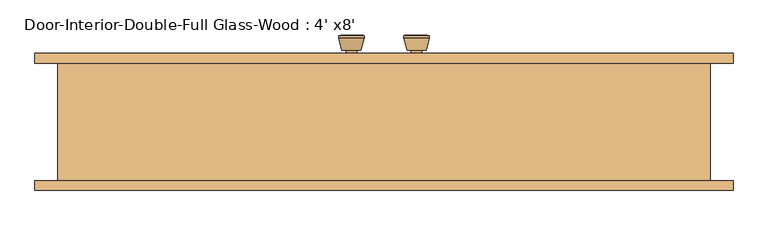
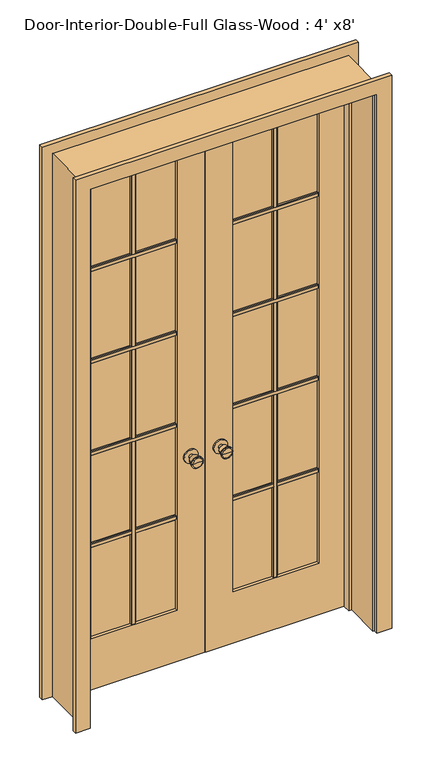
"""IFC4 building model written with IfcOpenShell, lengths in millimetres: door geometry, Door-Interior-Double-Full Glass-Wood : 4' x8'."""

from ifc_helpers import new_model, si_unit, point, frame, frame_2d, origin, place, context, project, spatial, polyline, circle_curve, trimmed, segment, composite_curve, outline, extrude, faceted_brep, source, transform, mapped, element, save
from ifc_brep_helpers import plane_surface, cylinder_surface, revolved_surface, advanced_brep


def door_interior_double_full_glass_wood_4_x8_0c92ad92(model_context):
    return source(origin(), model_context, "Body", "SolidModel", [
        advanced_brep(
        [(-63.5, 117.125, 914.4), (-73.5, 117.125, 914.4), (-53.5, 117.125, 914.4), (-83.9758676, 166.125, 914.4), (-63.5, 166.125, 914.4), (-43.0241324, 166.125, 914.4), (-88.5, 164.2971319, 914.4), (-38.5, 164.2971319, 914.4), (-88.5, 160.8334537, 914.4), (-38.5, 160.8334537, 914.4), (-82.136236, 136.125, 914.4), (-44.863764, 136.125, 914.4), (-73.5, 136.125, 914.4), (-53.5, 136.125, 914.4)],
        [
            (0, 1),
            (1, 2, circle_curve(frame((-63.5, 117.125, 914.4), z_axis=(0.0, -1.0, 0.0), x_axis=(1.0, 0.0, 0.0)), 10.0)),
            (2, 0),
            (2, 1, circle_curve(frame((-63.5, 117.125, 914.4), z_axis=(0.0, -1.0, 0.0), x_axis=(1.0, 0.0, 0.0)), 10.0)),
            (3, 4),
            (4, 5),
            (5, 3, circle_curve(frame((-63.5, 166.125, 914.4), z_axis=(0.0, 1.0, 0.0), x_axis=(1.0, 0.0, 0.0)), 20.4758676)),
            (3, 5, circle_curve(frame((-63.5, 166.125, 914.4), z_axis=(0.0, 1.0, 0.0), x_axis=(1.0, 0.0, 0.0)), 20.4758676)),
            (6, 3),
            (5, 7),
            (7, 6, circle_curve(frame((-63.5, 164.2971319, 914.4), z_axis=(0.0, 1.0, 0.0), x_axis=(1.0, 0.0, 0.0)), 25.0)),
            (6, 7, circle_curve(frame((-63.5, 164.2971319, 914.4), z_axis=(0.0, 1.0, 0.0), x_axis=(1.0, 0.0, 0.0)), 25.0)),
            (8, 6),
            (7, 9),
            (9, 8, circle_curve(frame((-63.5, 160.8334537, 914.4), z_axis=(0.0, 1.0, 0.0), x_axis=(1.0, 0.0, 0.0)), 25.0)),
            (8, 9, circle_curve(frame((-63.5, 160.8334537, 914.4), z_axis=(0.0, 1.0, 0.0), x_axis=(1.0, 0.0, 0.0)), 25.0)),
            (10, 8),
            (9, 11),
            (11, 10, circle_curve(frame((-63.5, 136.125, 914.4), z_axis=(0.0, 1.0, 0.0), x_axis=(1.0, 0.0, 0.0)), 18.636236)),
            (10, 11, circle_curve(frame((-63.5, 136.125, 914.4), z_axis=(0.0, 1.0, 0.0), x_axis=(1.0, 0.0, 0.0)), 18.636236)),
            (12, 10),
            (11, 13),
            (13, 12, circle_curve(frame((-63.5, 136.125, 914.4), z_axis=(0.0, 1.0, 0.0), x_axis=(1.0, 0.0, 0.0)), 10.0)),
            (12, 13, circle_curve(frame((-63.5, 136.125, 914.4), z_axis=(0.0, 1.0, 0.0), x_axis=(1.0, 0.0, 0.0)), 10.0)),
            (1, 12),
            (13, 2),
        ],
        [
            plane_surface(frame((-63.5, 117.125, 914.4), z_axis=(0.0, -1.0, 0.0), x_axis=(1.0, 0.0, 0.0))),
            plane_surface(frame((-63.5, 166.125, 914.4), z_axis=(0.0, 1.0, 0.0), x_axis=(1.0, 0.0, 0.0))),
            revolved_surface(polyline([(-43.0241324, 166.125, 914.4), (-38.5, 164.2971319, 914.4)]), (-63.5, 117.125, 914.4), (0.0, -1.0, 0.0)),
            cylinder_surface(frame((-63.5, 117.125, 914.4), z_axis=(0.0, -1.0, 0.0), x_axis=(1.0, 0.0, 0.0)), 25.0),
            revolved_surface(polyline([(-38.5, 160.8334537, 914.4), (-44.863764, 136.125, 914.4)]), (-63.5, 117.125, 914.4), (0.0, -1.0, 0.0)),
            plane_surface(frame((-63.5, 136.125, 914.4), z_axis=(0.0, -1.0, 0.0), x_axis=(1.0, 0.0, 0.0))),
            cylinder_surface(frame((-63.5, 117.125, 914.4), z_axis=(0.0, -1.0, 0.0), x_axis=(1.0, 0.0, 0.0)), 10.0),
        ],
        [
            (0, [[1, 2, 3]]),
            (0, [[-3, 4, -1]]),
            (1, [[5, 6, 7]]),
            (1, [[-6, -5, 8]]),
            (2, [[9, -7, 10, 11]]),
            (2, [[-10, -8, -9, 12]]),
            (3, [[13, -11, 14, 15]]),
            (3, [[-14, -12, -13, 16]]),
            (4, [[17, -15, 18, 19]]),
            (4, [[-18, -16, -17, 20]]),
            (5, [[21, -19, 22, 23]]),
            (5, [[-22, -20, -21, 24]]),
            (6, [[25, -23, 26, -2]]),
            (6, [[-26, -24, -25, -4]]),
        ],
    ),
        extrude(outline(composite_curve([segment(trimmed(circle_curve(frame_2d((914.4, -63.5)), 30.0), [point((914.4, -33.5))], [point((914.4, -93.5))], False, "CARTESIAN"), True, "CONTINUOUS"), segment(trimmed(circle_curve(frame_2d((914.4, -63.5)), 30.0), [point((914.4, -93.5))], [point((914.4, -33.5))], False, "CARTESIAN"), True, "CONTINUOUS")], self_intersect=False)), frame((0.0, 111.125, 0.0), z_axis=(0.0, 1.0, 0.0), x_axis=(0.0, 0.0, 1.0)), (0.0, 0.0, 1.0), 6.0),
        advanced_brep(
        [(-63.5, 70.2, 914.4), (-53.5, 70.2, 914.4), (-73.5, 70.2, 914.4), (-83.9758676, 21.2, 914.4), (-43.0241324, 21.2, 914.4), (-63.5, 21.2, 914.4), (-88.5, 23.0278681, 914.4), (-38.5, 23.0278681, 914.4), (-88.5, 26.4915463, 914.4), (-38.5, 26.4915463, 914.4), (-82.136236, 51.2, 914.4), (-44.863764, 51.2, 914.4), (-73.5, 51.2, 914.4), (-53.5, 51.2, 914.4)],
        [
            (0, 1),
            (1, 2, circle_curve(frame((-63.5, 70.2, 914.4), z_axis=(0.0, 1.0, 0.0), x_axis=(1.0, 0.0, 0.0)), 10.0)),
            (2, 0),
            (2, 1, circle_curve(frame((-63.5, 70.2, 914.4), z_axis=(0.0, 1.0, 0.0), x_axis=(1.0, 0.0, 0.0)), 10.0)),
            (3, 4, circle_curve(frame((-63.5, 21.2, 914.4), z_axis=(0.0, -1.0, 0.0), x_axis=(1.0, 0.0, 0.0)), 20.4758676)),
            (4, 5),
            (5, 3),
            (4, 3, circle_curve(frame((-63.5, 21.2, 914.4), z_axis=(0.0, -1.0, 0.0), x_axis=(1.0, 0.0, 0.0)), 20.4758676)),
            (6, 7, circle_curve(frame((-63.5, 23.0278681, 914.4), z_axis=(0.0, -1.0, 0.0), x_axis=(1.0, 0.0, 0.0)), 25.0)),
            (7, 4),
            (3, 6),
            (7, 6, circle_curve(frame((-63.5, 23.0278681, 914.4), z_axis=(0.0, -1.0, 0.0), x_axis=(1.0, 0.0, 0.0)), 25.0)),
            (8, 9, circle_curve(frame((-63.5, 26.4915463, 914.4), z_axis=(0.0, -1.0, 0.0), x_axis=(1.0, 0.0, 0.0)), 25.0)),
            (9, 7),
            (6, 8),
            (9, 8, circle_curve(frame((-63.5, 26.4915463, 914.4), z_axis=(0.0, -1.0, 0.0), x_axis=(1.0, 0.0, 0.0)), 25.0)),
            (10, 11, circle_curve(frame((-63.5, 51.2, 914.4), z_axis=(0.0, -1.0, 0.0), x_axis=(1.0, 0.0, 0.0)), 18.636236)),
            (11, 9),
            (8, 10),
            (11, 10, circle_curve(frame((-63.5, 51.2, 914.4), z_axis=(0.0, -1.0, 0.0), x_axis=(1.0, 0.0, 0.0)), 18.636236)),
            (12, 13, circle_curve(frame((-63.5, 51.2, 914.4), z_axis=(0.0, -1.0, 0.0), x_axis=(1.0, 0.0, 0.0)), 10.0)),
            (13, 11),
            (10, 12),
            (13, 12, circle_curve(frame((-63.5, 51.2, 914.4), z_axis=(0.0, -1.0, 0.0), x_axis=(1.0, 0.0, 0.0)), 10.0)),
            (1, 13),
            (12, 2),
        ],
        [
            plane_surface(frame((-63.5, 70.2, 914.4), z_axis=(0.0, 1.0, 0.0), x_axis=(1.0, 0.0, 0.0))),
            plane_surface(frame((-63.5, 21.2, 914.4), z_axis=(0.0, -1.0, 0.0), x_axis=(1.0, 0.0, 0.0))),
            revolved_surface(polyline([(-43.0241324, 21.2, 914.4), (-38.5, 23.0278681, 914.4)]), (-63.5, 70.2, 914.4), (0.0, 1.0, 0.0)),
            cylinder_surface(frame((-63.5, 70.2, 914.4), z_axis=(0.0, 1.0, 0.0), x_axis=(1.0, 0.0, 0.0)), 25.0),
            revolved_surface(polyline([(-38.5, 26.4915463, 914.4), (-44.863764, 51.2, 914.4)]), (-63.5, 70.2, 914.4), (0.0, 1.0, 0.0)),
            plane_surface(frame((-63.5, 51.2, 914.4), z_axis=(0.0, 1.0, 0.0), x_axis=(1.0, 0.0, 0.0))),
            cylinder_surface(frame((-63.5, 70.2, 914.4), z_axis=(0.0, 1.0, 0.0), x_axis=(1.0, 0.0, 0.0)), 10.0),
        ],
        [
            (0, [[1, 2, 3]]),
            (0, [[-3, 4, -1]]),
            (1, [[5, 6, 7]]),
            (1, [[8, -7, -6]]),
            (2, [[9, 10, -5, 11]]),
            (2, [[12, -11, -8, -10]]),
            (3, [[13, 14, -9, 15]]),
            (3, [[16, -15, -12, -14]]),
            (4, [[17, 18, -13, 19]]),
            (4, [[20, -19, -16, -18]]),
            (5, [[21, 22, -17, 23]]),
            (5, [[24, -23, -20, -22]]),
            (6, [[-2, 25, -21, 26]]),
            (6, [[-4, -26, -24, -25]]),
        ],
    ),
        extrude(outline(composite_curve([segment(trimmed(circle_curve(frame_2d((914.4, -63.5)), 30.0), [point((914.4, -33.5))], [point((914.4, -93.5))], False, "CARTESIAN"), True, "CONTINUOUS"), segment(trimmed(circle_curve(frame_2d((914.4, -63.5)), 30.0), [point((914.4, -93.5))], [point((914.4, -33.5))], False, "CARTESIAN"), True, "CONTINUOUS")], self_intersect=False)), frame((0.0, 70.2, 0.0), z_axis=(0.0, 1.0, 0.0), x_axis=(0.0, 0.0, 1.0)), (0.0, 0.0, 1.0), 6.0),
        extrude(outline(polyline([(90.17, 1911.35), (90.17, 1892.3), (83.82, 1892.3), (80.645, 1895.475), (80.645, 1908.175), (83.82, 1911.35), (90.17, 1911.35)])), frame((120.65, 0.0, 0.0), z_axis=(1.0, 0.0, 0.0), x_axis=(0.0, 1.0, 0.0)), (0.0, 0.0, 1.0), 368.3),
        extrude(outline(polyline([(90.17, 1493.8375), (90.17, 1474.7875), (83.82, 1474.7875), (80.645, 1477.9625), (80.645, 1490.6625), (83.82, 1493.8375), (90.17, 1493.8375)])), frame((120.65, 0.0, 0.0), z_axis=(1.0, 0.0, 0.0), x_axis=(0.0, 1.0, 0.0)), (0.0, 0.0, 1.0), 368.3),
        extrude(outline(polyline([(90.17, 1076.325), (90.17, 1057.275), (83.82, 1057.275), (80.645, 1060.45), (80.645, 1073.15), (83.82, 1076.325), (90.17, 1076.325)])), frame((120.65, 0.0, 0.0), z_axis=(1.0, 0.0, 0.0), x_axis=(0.0, 1.0, 0.0)), (0.0, 0.0, 1.0), 368.3),
        extrude(outline(polyline([(295.275, 90.17), (314.325, 90.17), (314.325, 83.82), (311.15, 80.645), (298.45, 80.645), (295.275, 83.82), (295.275, 90.17)])), frame((0.0, 0.0, 231.775), z_axis=(0.0, 0.0, 1.0), x_axis=(1.0, 0.0, 0.0)), (0.0, 0.0, 1.0), 2087.5625),
        extrude(outline(polyline([(90.17, 658.8125), (90.17, 639.7625), (83.82, 639.7625), (80.645, 642.9375), (80.645, 655.6375), (83.82, 658.8125), (90.17, 658.8125)])), frame((120.65, 0.0, 0.0), z_axis=(1.0, 0.0, 0.0), x_axis=(0.0, 1.0, 0.0)), (0.0, 0.0, 1.0), 368.3),
        extrude(outline(polyline([(97.155, 1911.35), (103.505, 1911.35), (106.68, 1908.175), (106.68, 1895.475), (103.505, 1892.3), (97.155, 1892.3), (97.155, 1911.35)])), frame((-488.95, 0.0, 0.0), z_axis=(1.0, 0.0, 0.0), x_axis=(0.0, 1.0, 0.0)), (0.0, 0.0, 1.0), 368.3),
        extrude(outline(polyline([(97.155, 1493.8375), (103.505, 1493.8375), (106.68, 1490.6625), (106.68, 1477.9625), (103.505, 1474.7875), (97.155, 1474.7875), (97.155, 1493.8375)])), frame((-488.95, 0.0, 0.0), z_axis=(1.0, 0.0, 0.0), x_axis=(0.0, 1.0, 0.0)), (0.0, 0.0, 1.0), 368.3),
        extrude(outline(polyline([(97.155, 1076.325), (103.505, 1076.325), (106.68, 1073.15), (106.68, 1060.45), (103.505, 1057.275), (97.155, 1057.275), (97.155, 1076.325)])), frame((-488.95, 0.0, 0.0), z_axis=(1.0, 0.0, 0.0), x_axis=(0.0, 1.0, 0.0)), (0.0, 0.0, 1.0), 368.3),
        extrude(outline(polyline([(-314.325, 97.155), (-314.325, 103.505), (-311.15, 106.68), (-298.45, 106.68), (-295.275, 103.505), (-295.275, 97.155), (-314.325, 97.155)])), frame((0.0, 0.0, 231.775), z_axis=(0.0, 0.0, 1.0), x_axis=(1.0, 0.0, 0.0)), (0.0, 0.0, 1.0), 2087.5625),
        extrude(outline(polyline([(97.155, 658.8125), (103.505, 658.8125), (106.68, 655.6375), (106.68, 642.9375), (103.505, 639.7625), (97.155, 639.7625), (97.155, 658.8125)])), frame((-488.95, 0.0, 0.0), z_axis=(1.0, 0.0, 0.0), x_axis=(0.0, 1.0, 0.0)), (0.0, 0.0, 1.0), 368.3),
        extrude(outline(polyline([(97.155, 1911.35), (103.505, 1911.35), (106.68, 1908.175), (106.68, 1895.475), (103.505, 1892.3), (97.155, 1892.3), (97.155, 1911.35)])), frame((120.65, 0.0, 0.0), z_axis=(1.0, 0.0, 0.0), x_axis=(0.0, 1.0, 0.0)), (0.0, 0.0, 1.0), 368.3),
        extrude(outline(polyline([(97.155, 1493.8375), (103.505, 1493.8375), (106.68, 1490.6625), (106.68, 1477.9625), (103.505, 1474.7875), (97.155, 1474.7875), (97.155, 1493.8375)])), frame((120.65, 0.0, 0.0), z_axis=(1.0, 0.0, 0.0), x_axis=(0.0, 1.0, 0.0)), (0.0, 0.0, 1.0), 368.3),
        extrude(outline(polyline([(97.155, 1076.325), (103.505, 1076.325), (106.68, 1073.15), (106.68, 1060.45), (103.505, 1057.275), (97.155, 1057.275), (97.155, 1076.325)])), frame((120.65, 0.0, 0.0), z_axis=(1.0, 0.0, 0.0), x_axis=(0.0, 1.0, 0.0)), (0.0, 0.0, 1.0), 368.3),
        extrude(outline(polyline([(295.275, 97.155), (295.275, 103.505), (298.45, 106.68), (311.15, 106.68), (314.325, 103.505), (314.325, 97.155), (295.275, 97.155)])), frame((0.0, 0.0, 231.775), z_axis=(0.0, 0.0, 1.0), x_axis=(1.0, 0.0, 0.0)), (0.0, 0.0, 1.0), 2087.5625),
        extrude(outline(polyline([(97.155, 658.8125), (103.505, 658.8125), (106.68, 655.6375), (106.68, 642.9375), (103.505, 639.7625), (97.155, 639.7625), (97.155, 658.8125)])), frame((120.65, 0.0, 0.0), z_axis=(1.0, 0.0, 0.0), x_axis=(0.0, 1.0, 0.0)), (0.0, 0.0, 1.0), 368.3),
        extrude(outline(polyline([(90.17, 1911.35), (90.17, 1892.3), (83.82, 1892.3), (80.645, 1895.475), (80.645, 1908.175), (83.82, 1911.35), (90.17, 1911.35)])), frame((-488.95, 0.0, 0.0), z_axis=(1.0, 0.0, 0.0), x_axis=(0.0, 1.0, 0.0)), (0.0, 0.0, 1.0), 368.3),
        extrude(outline(polyline([(90.17, 1493.8375), (90.17, 1474.7875), (83.82, 1474.7875), (80.645, 1477.9625), (80.645, 1490.6625), (83.82, 1493.8375), (90.17, 1493.8375)])), frame((-488.95, 0.0, 0.0), z_axis=(1.0, 0.0, 0.0), x_axis=(0.0, 1.0, 0.0)), (0.0, 0.0, 1.0), 368.3),
        extrude(outline(polyline([(90.17, 1076.325), (90.17, 1057.275), (83.82, 1057.275), (80.645, 1060.45), (80.645, 1073.15), (83.82, 1076.325), (90.17, 1076.325)])), frame((-488.95, 0.0, 0.0), z_axis=(1.0, 0.0, 0.0), x_axis=(0.0, 1.0, 0.0)), (0.0, 0.0, 1.0), 368.3),
        extrude(outline(polyline([(-314.325, 90.17), (-295.275, 90.17), (-295.275, 83.82), (-298.45, 80.645), (-311.15, 80.645), (-314.325, 83.82), (-314.325, 90.17)])), frame((0.0, 0.0, 231.775), z_axis=(0.0, 0.0, 1.0), x_axis=(1.0, 0.0, 0.0)), (0.0, 0.0, 1.0), 2087.5625),
        extrude(outline(polyline([(90.17, 658.8125), (90.17, 639.7625), (83.82, 639.7625), (80.645, 642.9375), (80.645, 655.6375), (83.82, 658.8125), (90.17, 658.8125)])), frame((-488.95, 0.0, 0.0), z_axis=(1.0, 0.0, 0.0), x_axis=(0.0, 1.0, 0.0)), (0.0, 0.0, 1.0), 368.3),
        advanced_brep(
        [(63.5, 70.2, 914.4), (73.5, 70.2, 914.4), (53.5, 70.2, 914.4), (83.9758676, 21.2, 914.4), (63.5, 21.2, 914.4), (43.0241324, 21.2, 914.4), (88.5, 23.0278681, 914.4), (38.5, 23.0278681, 914.4), (88.5, 26.4915463, 914.4), (38.5, 26.4915463, 914.4), (82.136236, 51.2, 914.4), (44.863764, 51.2, 914.4), (73.5, 51.2, 914.4), (53.5, 51.2, 914.4)],
        [
            (0, 1),
            (1, 2, circle_curve(frame((63.5, 70.2, 914.4), z_axis=(0.0, 1.0, 0.0), x_axis=(-1.0, 0.0, 0.0)), 10.0)),
            (2, 0),
            (2, 1, circle_curve(frame((63.5, 70.2, 914.4), z_axis=(0.0, 1.0, 0.0), x_axis=(-1.0, 0.0, 0.0)), 10.0)),
            (3, 4),
            (4, 5),
            (5, 3, circle_curve(frame((63.5, 21.2, 914.4), z_axis=(0.0, -1.0, 0.0), x_axis=(-1.0, 0.0, 0.0)), 20.4758676)),
            (3, 5, circle_curve(frame((63.5, 21.2, 914.4), z_axis=(0.0, -1.0, 0.0), x_axis=(-1.0, 0.0, 0.0)), 20.4758676)),
            (6, 3),
            (5, 7),
            (7, 6, circle_curve(frame((63.5, 23.0278681, 914.4), z_axis=(0.0, -1.0, 0.0), x_axis=(-1.0, 0.0, 0.0)), 25.0)),
            (6, 7, circle_curve(frame((63.5, 23.0278681, 914.4), z_axis=(0.0, -1.0, 0.0), x_axis=(-1.0, 0.0, 0.0)), 25.0)),
            (8, 6),
            (7, 9),
            (9, 8, circle_curve(frame((63.5, 26.4915463, 914.4), z_axis=(0.0, -1.0, 0.0), x_axis=(-1.0, 0.0, 0.0)), 25.0)),
            (8, 9, circle_curve(frame((63.5, 26.4915463, 914.4), z_axis=(0.0, -1.0, 0.0), x_axis=(-1.0, 0.0, 0.0)), 25.0)),
            (10, 8),
            (9, 11),
            (11, 10, circle_curve(frame((63.5, 51.2, 914.4), z_axis=(0.0, -1.0, 0.0), x_axis=(-1.0, 0.0, 0.0)), 18.636236)),
            (10, 11, circle_curve(frame((63.5, 51.2, 914.4), z_axis=(0.0, -1.0, 0.0), x_axis=(-1.0, 0.0, 0.0)), 18.636236)),
            (12, 10),
            (11, 13),
            (13, 12, circle_curve(frame((63.5, 51.2, 914.4), z_axis=(0.0, -1.0, 0.0), x_axis=(-1.0, 0.0, 0.0)), 10.0)),
            (12, 13, circle_curve(frame((63.5, 51.2, 914.4), z_axis=(0.0, -1.0, 0.0), x_axis=(-1.0, 0.0, 0.0)), 10.0)),
            (1, 12),
            (13, 2),
        ],
        [
            plane_surface(frame((63.5, 70.2, 914.4), z_axis=(0.0, 1.0, 0.0), x_axis=(-1.0, 0.0, 0.0))),
            plane_surface(frame((63.5, 21.2, 914.4), z_axis=(0.0, -1.0, 0.0), x_axis=(-1.0, 0.0, 0.0))),
            revolved_surface(polyline([(43.0241324, 21.2, 914.4), (38.5, 23.0278681, 914.4)]), (63.5, 70.2, 914.4), (0.0, 1.0, 0.0)),
            cylinder_surface(frame((63.5, 70.2, 914.4), z_axis=(0.0, 1.0, 0.0), x_axis=(-1.0, 0.0, 0.0)), 25.0),
            revolved_surface(polyline([(38.5, 26.4915463, 914.4), (44.863764, 51.2, 914.4)]), (63.5, 70.2, 914.4), (0.0, 1.0, 0.0)),
            plane_surface(frame((63.5, 51.2, 914.4), z_axis=(0.0, 1.0, 0.0), x_axis=(-1.0, 0.0, 0.0))),
            cylinder_surface(frame((63.5, 70.2, 914.4), z_axis=(0.0, 1.0, 0.0), x_axis=(-1.0, 0.0, 0.0)), 10.0),
        ],
        [
            (0, [[1, 2, 3]]),
            (0, [[-3, 4, -1]]),
            (1, [[5, 6, 7]]),
            (1, [[-6, -5, 8]]),
            (2, [[9, -7, 10, 11]]),
            (2, [[-10, -8, -9, 12]]),
            (3, [[13, -11, 14, 15]]),
            (3, [[-14, -12, -13, 16]]),
            (4, [[17, -15, 18, 19]]),
            (4, [[-18, -16, -17, 20]]),
            (5, [[21, -19, 22, 23]]),
            (5, [[-22, -20, -21, 24]]),
            (6, [[25, -23, 26, -2]]),
            (6, [[-26, -24, -25, -4]]),
        ],
    ),
        extrude(outline(composite_curve([segment(trimmed(circle_curve(frame_2d((914.4, 63.5)), 30.0), [point((914.4, 33.5))], [point((914.4, 93.5))], False, "CARTESIAN"), True, "CONTINUOUS"), segment(trimmed(circle_curve(frame_2d((914.4, 63.5)), 30.0), [point((914.4, 93.5))], [point((914.4, 33.5))], False, "CARTESIAN"), True, "CONTINUOUS")], self_intersect=False)), frame((0.0, 70.2, 0.0), z_axis=(0.0, 1.0, 0.0), x_axis=(0.0, 0.0, 1.0)), (0.0, 0.0, 1.0), 6.0),
        advanced_brep(
        [(63.5, 117.125, 914.4), (53.5, 117.125, 914.4), (73.5, 117.125, 914.4), (83.9758676, 166.125, 914.4), (43.0241324, 166.125, 914.4), (63.5, 166.125, 914.4), (88.5, 164.2971319, 914.4), (38.5, 164.2971319, 914.4), (88.5, 160.8334537, 914.4), (38.5, 160.8334537, 914.4), (82.136236, 136.125, 914.4), (44.863764, 136.125, 914.4), (73.5, 136.125, 914.4), (53.5, 136.125, 914.4)],
        [
            (0, 1),
            (1, 2, circle_curve(frame((63.5, 117.125, 914.4), z_axis=(0.0, -1.0, 0.0), x_axis=(-1.0, 0.0, 0.0)), 10.0)),
            (2, 0),
            (2, 1, circle_curve(frame((63.5, 117.125, 914.4), z_axis=(0.0, -1.0, 0.0), x_axis=(-1.0, 0.0, 0.0)), 10.0)),
            (3, 4, circle_curve(frame((63.5, 166.125, 914.4), z_axis=(0.0, 1.0, 0.0), x_axis=(-1.0, 0.0, 0.0)), 20.4758676)),
            (4, 5),
            (5, 3),
            (4, 3, circle_curve(frame((63.5, 166.125, 914.4), z_axis=(0.0, 1.0, 0.0), x_axis=(-1.0, 0.0, 0.0)), 20.4758676)),
            (6, 7, circle_curve(frame((63.5, 164.2971319, 914.4), z_axis=(0.0, 1.0, 0.0), x_axis=(-1.0, 0.0, 0.0)), 25.0)),
            (7, 4),
            (3, 6),
            (7, 6, circle_curve(frame((63.5, 164.2971319, 914.4), z_axis=(0.0, 1.0, 0.0), x_axis=(-1.0, 0.0, 0.0)), 25.0)),
            (8, 9, circle_curve(frame((63.5, 160.8334537, 914.4), z_axis=(0.0, 1.0, 0.0), x_axis=(-1.0, 0.0, 0.0)), 25.0)),
            (9, 7),
            (6, 8),
            (9, 8, circle_curve(frame((63.5, 160.8334537, 914.4), z_axis=(0.0, 1.0, 0.0), x_axis=(-1.0, 0.0, 0.0)), 25.0)),
            (10, 11, circle_curve(frame((63.5, 136.125, 914.4), z_axis=(0.0, 1.0, 0.0), x_axis=(-1.0, 0.0, 0.0)), 18.636236)),
            (11, 9),
            (8, 10),
            (11, 10, circle_curve(frame((63.5, 136.125, 914.4), z_axis=(0.0, 1.0, 0.0), x_axis=(-1.0, 0.0, 0.0)), 18.636236)),
            (12, 13, circle_curve(frame((63.5, 136.125, 914.4), z_axis=(0.0, 1.0, 0.0), x_axis=(-1.0, 0.0, 0.0)), 10.0)),
            (13, 11),
            (10, 12),
            (13, 12, circle_curve(frame((63.5, 136.125, 914.4), z_axis=(0.0, 1.0, 0.0), x_axis=(-1.0, 0.0, 0.0)), 10.0)),
            (1, 13),
            (12, 2),
        ],
        [
            plane_surface(frame((63.5, 117.125, 914.4), z_axis=(0.0, -1.0, 0.0), x_axis=(-1.0, 0.0, 0.0))),
            plane_surface(frame((63.5, 166.125, 914.4), z_axis=(0.0, 1.0, 0.0), x_axis=(-1.0, 0.0, 0.0))),
            revolved_surface(polyline([(43.0241324, 166.125, 914.4), (38.5, 164.2971319, 914.4)]), (63.5, 117.125, 914.4), (0.0, -1.0, 0.0)),
            cylinder_surface(frame((63.5, 117.125, 914.4), z_axis=(0.0, -1.0, 0.0), x_axis=(-1.0, 0.0, 0.0)), 25.0),
            revolved_surface(polyline([(38.5, 160.8334537, 914.4), (44.863764, 136.125, 914.4)]), (63.5, 117.125, 914.4), (0.0, -1.0, 0.0)),
            plane_surface(frame((63.5, 136.125, 914.4), z_axis=(0.0, -1.0, 0.0), x_axis=(-1.0, 0.0, 0.0))),
            cylinder_surface(frame((63.5, 117.125, 914.4), z_axis=(0.0, -1.0, 0.0), x_axis=(-1.0, 0.0, 0.0)), 10.0),
        ],
        [
            (0, [[1, 2, 3]]),
            (0, [[-3, 4, -1]]),
            (1, [[5, 6, 7]]),
            (1, [[8, -7, -6]]),
            (2, [[9, 10, -5, 11]]),
            (2, [[12, -11, -8, -10]]),
            (3, [[13, 14, -9, 15]]),
            (3, [[16, -15, -12, -14]]),
            (4, [[17, 18, -13, 19]]),
            (4, [[20, -19, -16, -18]]),
            (5, [[21, 22, -17, 23]]),
            (5, [[24, -23, -20, -22]]),
            (6, [[-2, 25, -21, 26]]),
            (6, [[-4, -26, -24, -25]]),
        ],
    ),
        extrude(outline(composite_curve([segment(trimmed(circle_curve(frame_2d((914.4, 63.5)), 30.0), [point((914.4, 33.5))], [point((914.4, 93.5))], False, "CARTESIAN"), True, "CONTINUOUS"), segment(trimmed(circle_curve(frame_2d((914.4, 63.5)), 30.0), [point((914.4, 93.5))], [point((914.4, 33.5))], False, "CARTESIAN"), True, "CONTINUOUS")], self_intersect=False)), frame((0.0, 111.125, 0.0), z_axis=(0.0, 1.0, 0.0), x_axis=(0.0, 0.0, 1.0)), (0.0, 0.0, 1.0), 6.0),
        extrude(outline(polyline([(0.0, 615.95), (0.0, 679.45), (2508.25, 679.45), (2508.25, -679.45), (0.0, -679.45), (0.0, -615.95), (2444.75, -615.95), (2444.75, 615.95), (0.0, 615.95)])), frame((0.0, -136.525, 0.0), z_axis=(0.0, 1.0, 0.0), x_axis=(0.0, 0.0, 1.0)), (0.0, 0.0, 1.0), 19.05),
        extrude(outline(polyline([(0.0, 615.95), (0.0, 679.45), (2508.25, 679.45), (2508.25, -679.45), (0.0, -679.45), (0.0, -615.95), (2444.75, -615.95), (2444.75, 615.95), (0.0, 615.95)])), frame((0.0, 111.125, 0.0), z_axis=(0.0, 1.0, 0.0), x_axis=(0.0, 0.0, 1.0)), (0.0, 0.0, 1.0), 19.05),
        faceted_brep([(635.0, 111.125, 0.0), (635.0, -117.475, 0.0), (609.6, -117.475, 0.0), (609.6, 41.275, 0.0), (596.9, 41.275, 0.0), (596.9, 76.2, 0.0), (609.6, 76.2, 0.0), (609.6, 111.125, 0.0), (635.0, 111.125, 2463.8), (635.0, -117.475, 2463.8), (-635.0, -117.475, 2463.8), (-635.0, -117.475, 0.0), (-609.6, -117.475, 0.0), (-609.6, -117.475, 2438.4), (609.6, -117.475, 2438.4), (609.6, 41.275, 2438.4), (-609.6, 41.275, 2438.4), (-609.6, 41.275, 0.0), (-596.9, 41.275, 0.0), (-596.9, 41.275, 2425.7), (596.9, 41.275, 2425.7), (596.9, 76.2, 2425.7), (1.5875, 76.2, 2425.7), (-1.6019111, 76.2, 2425.7), (-596.9, 76.2, 2425.7), (-596.9, 76.2, 0.0), (-609.6, 76.2, 0.0), (-609.6, 76.2, 2438.4), (-1.6019111, 76.2, 2438.4), (1.5875, 76.2, 2438.4), (609.6, 76.2, 2438.4), (609.6, 111.125, 2438.4), (1.5875, 111.125, 2438.4), (-1.6019111, 111.125, 2438.4), (-609.6, 111.125, 2438.4), (-609.6, 111.125, 0.0), (-635.0, 111.125, 0.0), (-635.0, 111.125, 2463.8)], [[[0, 1, 2, 3, 4, 5, 6, 7]], [[1, 0, 8, 9]], [[2, 1, 9, 10, 11, 12, 13, 14]], [[3, 2, 14, 15]], [[4, 3, 15, 16, 17, 18, 19, 20]], [[5, 4, 20, 21]], [[6, 5, 21, 22, 23, 24, 25, 26, 27, 28, 29, 30]], [[7, 6, 30, 31]], [[0, 7, 31, 32, 33, 34, 35, 36, 37, 8]], [[9, 8, 37, 10]], [[14, 13, 16, 15]], [[20, 19, 24, 23, 22, 21]], [[31, 30, 29, 28, 27, 34, 33, 32]], [[12, 11, 36, 35, 26, 25, 18, 17]], [[11, 10, 37, 36]], [[13, 12, 17, 16]], [[19, 18, 25, 24]], [[27, 26, 35, 34]]]),
        extrude(outline(polyline([(2438.4, -609.6), (0.0, -609.6), (0.0, -1.6019111), (2438.4, -1.6019111), (2438.4, -609.6)]), holes=[polyline([(231.775, -488.95), (2319.3375, -488.95), (2319.3375, -120.65), (231.775, -120.65), (231.775, -488.95)])]), frame((0.0, 76.2, 0.0), z_axis=(0.0, 1.0, 0.0), x_axis=(0.0, 0.0, 1.0)), (0.0, 0.0, 1.0), 34.925),
        extrude(outline(polyline([(0.0, 609.6), (2438.4, 609.6), (2438.4, 1.5875), (0.0, 1.5875), (0.0, 609.6)]), holes=[polyline([(2319.3375, 120.65), (2319.3375, 488.95), (231.775, 488.95), (231.775, 120.65), (2319.3375, 120.65)])]), frame((0.0, 76.2, 0.0), z_axis=(0.0, 1.0, 0.0), x_axis=(0.0, 0.0, 1.0)), (0.0, 0.0, 1.0), 34.925),
        extrude(outline(polyline([(488.95, 90.17), (120.65, 90.17), (120.65, 97.155), (488.95, 97.155), (488.95, 90.17)])), frame((0.0, 0.0, 231.775), z_axis=(0.0, 0.0, 1.0), x_axis=(1.0, 0.0, 0.0)), (0.0, 0.0, 1.0), 2087.5625),
        extrude(outline(polyline([(-120.65, 90.17), (-488.95, 90.17), (-488.95, 97.155), (-120.65, 97.155), (-120.65, 90.17)])), frame((0.0, 0.0, 231.775), z_axis=(0.0, 0.0, 1.0), x_axis=(1.0, 0.0, 0.0)), (0.0, 0.0, 1.0), 2087.5625),
    ])


if __name__ == "__main__":
    model = new_model("IFC4")
    model_context = context("Model", 3, world=origin())
    ifc_project = project(units=[si_unit("LENGTHUNIT", "METRE", prefix="MILLI")], contexts=[model_context])
    site = spatial("IfcSite", under=ifc_project)
    building = spatial("IfcBuilding", under=site)
    placement = place(None, origin())
    door_interior_double_full_glass_wood_4_x8_shape = door_interior_double_full_glass_wood_4_x8_0c92ad92(model_context)
    element("IfcDoor", 1, ObjectType="Door-Interior-Double-Full Glass-Wood : 4' x8'", at=placement, inside=building, context=model_context, shape_type="MappedRepresentation", body=[
        mapped(door_interior_double_full_glass_wood_4_x8_shape, transform((0.0, 0.0, 0.0), x_axis=(1.0, 0.0, 0.0), y_axis=(0.0, 1.0, 0.0), z_axis=(0.0, 0.0, 1.0))),
    ])
    save(model, "model.ifc")

# Revit data of these elements
# Type "Door-Interior-Double-Full Glass-Wood : 4' x8'"
#   Type Mark = "14"
#   Assembly Code = "C1020300"
#   Analytic Construction = "French door, wood frame with single glass"
#   Top Rail = 0' - 4 11/16"
#   Thickness = 0' - 1 3/8"
#   Thermal Resistance (R) = 1.0696 (h·ft²·°F)/BTU
#   Swing Angle [instance default] = 90.00°
#   Stiles = 0' - 4 3/4"
#   Rough Width = 4' - 2"
#   Rough Height = 8' - 1"
#   Panel Width = 2' - 0"
#   Height = 8' - 0"
#   Width = 4' - 0"
#   Heat Transfer Coefficient (U) = 0.9350 BTU/(h·ft²·°F)
#   Bottom Rail = 0' - 9 1/8"
#   Show Grill [instance default] = yes
#   Trim Material = Cherry
#   Panel Material = Cherry
#   Frame Material = Cherry
#   Door Handle Material = Aluminum
#   Visual Light Transmittance = 0
#   Solar Heat Gain Coefficient = 0
#   Wall Closure = (empty or 0)
#   Function = (empty or 0)
# Element 1 (IfcDoor, "Door-Interior-Double-Full Glass-Wood : 4' x8'")
#   Swing Angle = 45.00°
#   Materials on its faces: "Cherry", "Aluminum", "Glass"
# Materials
#   "Cherry": class "Wood", colour RGB 226 177 128, transparency 0, Description = "Prunus Serotina", Cost = 0
#   "Aluminum": class "Metal", colour RGB 247 247 247, transparency 0, Description = "Aluminum 6061", Cost = 0
#   "Glass": class "Glass", colour RGB 0 128 192, transparency 0.75, Description = "Soda Lime Glass", Cost = 0
